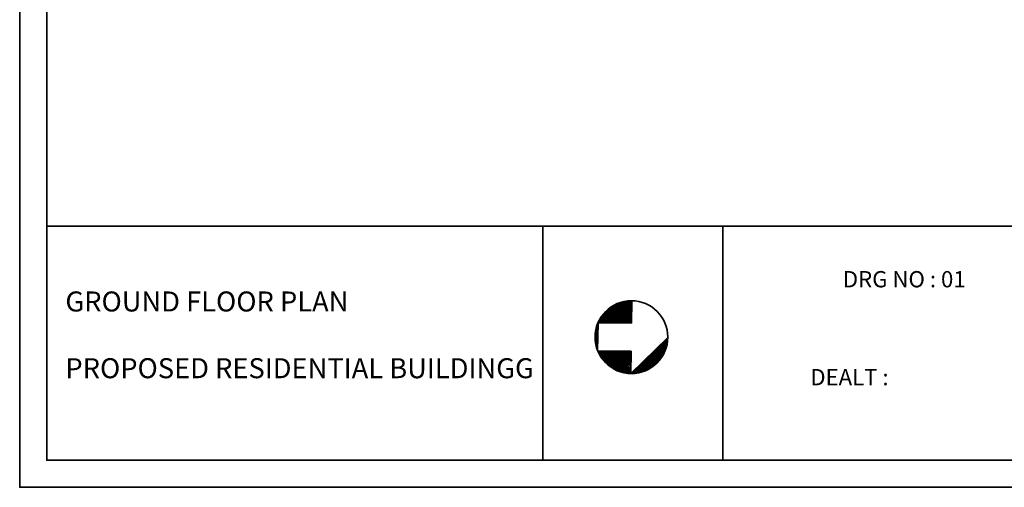
# Model space of a CAD drawing. Units: inches. Extents: x 1077 to 2505, y 1892 to 2728.
# Tile 1 of 26: x 1104 to 1433, y 1892 to 2048. Entities that reach past the tile are written whole.
import ezdxf

# ---------------------------------------------------------------- set-up
doc = ezdxf.new("R2010")
doc.units = ezdxf.units.IN
for name, color, linetype, lineweight in [('A-ANNO-SYMB', 18, 'Continuous', 18), ('A-ANNO-TTLB', 7, 'Continuous', 35), ('A_TEXT_SMALL', 18, 'Continuous', 13), ('walls', 250, 'Continuous', 35)]:
    doc.layers.add(name, color=color, linetype=linetype, lineweight=lineweight)
doc.styles.add('1-100DIM', font='txt', dxfattribs={"height": 0.3})

# ---------------------------------------------------------------- blocks, each defined once
blk = doc.blocks.new('NORTH')
at = {"layer": 'walls'}
h = blk.add_hatch(dxfattribs=at)
h.set_pattern_fill('ANSI31', color=256, scale=6.087211)
h.set_pattern_definition([(45, (-41048.0969, 128612.4242), (-0.53803848, 0.53803848), [])])
h.paths.add_polyline_path([(6704.42, -25696.22), (6687.22, -25696.22, 0.302843), (6704.42, -25722.01)])
h.paths.add_polyline_path([(6743.1, -25696.22), (6725.9, -25696.22), (6725.9, -25722.01, 0.302843)])
h.paths.add_polyline_path([(6715.16, -25668.28), (6743.1, -25696.22, 0.414214)])
h.paths.add_polyline_path([(6725.9, -25722.01), (6704.42, -25722.01, 0.199872)])
for p, q in [((6743.1, -25696.22, 0.29), (6715.16, -25668.28, 0.29)), ((6687.22, -25696.22, 0.29), (6704.42, -25696.22, 0.29)), ((6704.42, -25722.01, 0.29), (6704.42, -25696.22, 0.29)), ((6725.9, -25722.01, 0.29), (6725.9, -25696.22, 0.29)), ((6725.9, -25696.22, 0.29), (6743.1, -25696.22, 0.29)), ((6704.42, -25722.01, 0.29), (6725.9, -25722.01, 0.29))]:
    blk.add_line(p, q, dxfattribs=at)
blk.add_circle((6715.16, -25696.22, 0.29), 27.94, dxfattribs=at)
blk = doc.blocks.new('SHEET-FRAME-RESIDENTIAL')
for p, q in [((9, 87.01), (534.52, 87.01)), ((174.45, 87.01), (174.45, 9)), ((234.45, 87.01), (234.45, 9))]:
    blk.add_line(p, q)
for points in [[(0, 830.04), (543.52, 830.04), (543.52, 0), (0, 0)], [(9, 821.04), (534.52, 821.04), (534.52, 9), (9, 9)]]:
    blk.add_lwpolyline(points, close=True)

msp = doc.modelspace()

# ---------------------------------------------------------------- block references
at = {"layer": 'A-ANNO-SYMB', "xscale": 0.4341621291417894, "yscale": 0.4341621291417894, "zscale": 0.4341621291417894, "rotation": 269.2509902977627}
msp.add_blockref('NORTH', (12501.7, 4711.71, -0.13), dxfattribs=at)
at = {"layer": 'A-ANNO-TTLB'}
msp.add_blockref('SHEET-FRAME-RESIDENTIAL', (1104.25, 1892.27), dxfattribs=at)

# ---------------------------------------------------------------- texts
at = {"layer": 'A_TEXT_SMALL', "attachment_point": 1, "style": '1-100DIM'}
for s, width, gutter_width, insert, char_height in [('{\\f@Malgun Gothic|b0|i0|c0|p34;DRG NO : 01}', 152.9967, 8.47, (1378.72, 1964.36), 5.4184), ('{\\f@Malgun Gothic|b0|i0|c0|p34;GROUND FLOOR PLAN  \\P\\PPROPOSED RESIDENTIAL BUILDINGG}', 159.0041, 13.96, (1119.49, 1957.56), 6.6726), ('{\\f@Malgun Gothic|b0|i0|c0|p34;DEALT :}', 152.9967, 8.47, (1367.87, 1931.7), 5.4184)]:
    msp.add_mtext_dynamic_manual_height_columns(s, width=width, gutter_width=gutter_width, heights=[0], dxfattribs=dict(at, insert=insert, char_height=char_height))

doc.saveas('drawing.dxf')
